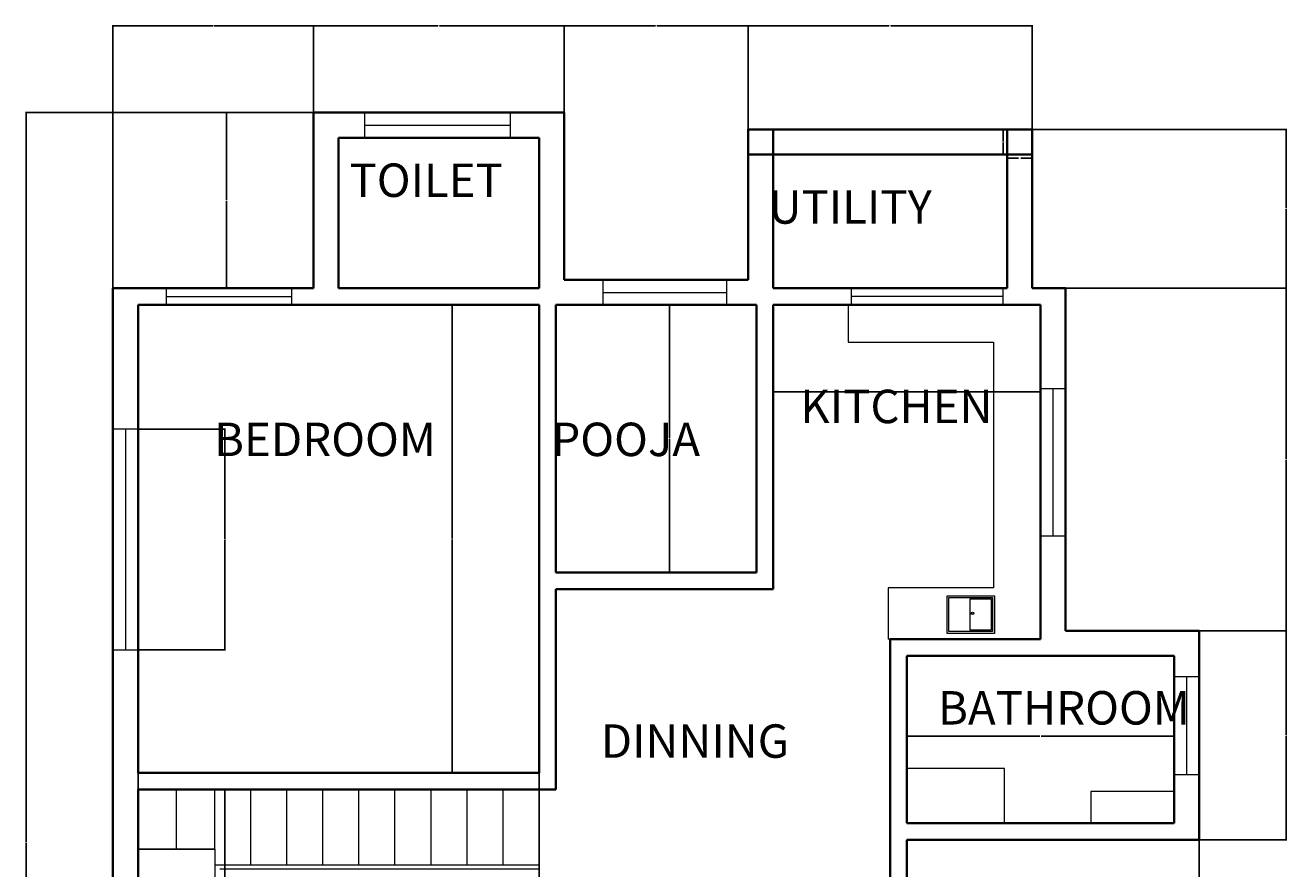
# Model space of a CAD drawing. Units: inches. Extents: x 1741 to 3812, y 9290 to 10023.
# Tile 2 of 5: x 1741 to 2194, y 9630 to 9933. Entities that reach past the tile are written whole.
import ezdxf

# ---------------------------------------------------------------- set-up
doc = ezdxf.new("R2010")
doc.units = ezdxf.units.IN
doc.header["$MEASUREMENT"] = 0
for name, color, linetype, lineweight in [('A-ANNO-DIMS', 2, 'Continuous', 18), ('A-AREA-IDEN', 7, 'Continuous', 18), ('A-COLS', 1, 'Continuous', 35), ('A-FLOR-CASE', 9, 'Continuous', 18), ('A-FLOR-FIXT', 8, 'Continuous', 18), ('A-FLOR-STRS', 3, 'Continuous', 18), ('A-GLAZ', 4, 'Continuous', 18), ('A-WALL', 7, 'Continuous', 35)]:
    doc.layers.add(name, color=color, linetype=linetype, lineweight=lineweight)
doc.styles.get("Standard").update_dxf_attribs({"font": 'arial.ttf'})
doc.dimstyles.get("Standard").update_dxf_attribs({"dimtxt": 0.18, "dimasz": 0.18, "dimexe": 0.18, "dimexo": 0.0625, "dimgap": 0.09, "dimtad": 0, "dimtih": 1, "dimtoh": 1, "dimdec": 4, "dimzin": 0, "dimdsep": 46, "dimtxsty": 'Standard', "dimcen": 0.09, "dimadec": 0, "dimazin": 0, "dimtfac": 1, "dimtdec": 4, "dimtofl": 0, "dimtmove": 0, "dimatfit": 3, "dimfxl": 1, "dimtolj": 1, "dimtzin": 0, "dimarcsym": 0})

# ---------------------------------------------------------------- blocks, each defined once
blk = doc.blocks.new('POST-9X9-PLAN')
blk.add_lwpolyline([(9, 0), (0, 0), (0, 9), (9, 9)], close=True)
blk = doc.blocks.new('*D15')
at = {"layer": 'A-ANNO-DIMS', "color": 0, "lineweight": -2, "transparency": 16777216}
for p, q in [((2093.86, 9895.45), (2092.39, 9895.45)), ((2092.57, 9895.27), (2092.57, 9891.13)), ((2092.57, 9886.63), (2092.57, 9890.77)), ((2093.86, 9886.45), (2092.39, 9886.45))]:
    blk.add_line(p, q, dxfattribs=at)
at = {"layer": 'A-ANNO-DIMS', "color": 0, "transparency": 16777216}
for points in [[(2092.54, 9895.27), (2092.6, 9895.27), (2092.57, 9895.45)], [(2092.54, 9886.63), (2092.6, 9886.63), (2092.57, 9886.45)]]:
    blk.add_solid(points, dxfattribs=at)
at = {"layer": 'Defpoints', "color": 0, "transparency": 16777216}
for p in [(2093.92, 9895.45), (2092.57, 9886.45), (2093.92, 9886.45)]:
    blk.add_point(p, dxfattribs=at)
at = {"layer": 'A-ANNO-DIMS', "color": 0, "transparency": 16777216, "insert": (2092.57, 9890.95), "char_height": 0.18, "attachment_point": 5}
blk.add_mtext('\\A1;POST 9 TYP.', dxfattribs=at)
blk = doc.blocks.new('*D16')
at = {"layer": 'A-ANNO-DIMS', "color": 0, "lineweight": -2, "transparency": 16777216}
for p, q in [((2093.92, 9886.39), (2093.92, 9884.92)), ((2094.1, 9885.1), (2097.97, 9885.1)), ((2102.74, 9885.1), (2098.88, 9885.1)), ((2102.92, 9886.39), (2102.92, 9884.92))]:
    blk.add_line(p, q, dxfattribs=at)
at = {"layer": 'A-ANNO-DIMS', "color": 0, "transparency": 16777216}
for points in [[(2094.1, 9885.13), (2094.1, 9885.07), (2093.92, 9885.1)], [(2102.74, 9885.13), (2102.74, 9885.07), (2102.92, 9885.1)]]:
    blk.add_solid(points, dxfattribs=at)
at = {"layer": 'Defpoints', "color": 0, "transparency": 16777216}
for p in [(2093.92, 9886.45), (2102.92, 9886.45), (2102.92, 9885.1)]:
    blk.add_point(p, dxfattribs=at)
at = {"layer": 'A-ANNO-DIMS', "color": 0, "transparency": 16777216, "insert": (2098.42, 9885.1), "char_height": 0.18, "attachment_point": 5}
blk.add_mtext('\\A1;9 TYP.', dxfattribs=at)
blk = doc.blocks.new('*D31')
at = {"layer": 'A-ANNO-DIMS', "color": 0, "lineweight": -2, "transparency": 16777216}
for p, q in [((2162.92, 9640.39), (2162.92, 9345.97)), ((1772.92, 9391.39), (1772.92, 9345.97)), ((1773.1, 9346.15), (1967.64, 9346.15)), ((2162.74, 9346.15), (1968.21, 9346.15))]:
    blk.add_line(p, q, dxfattribs=at)
at = {"layer": 'A-ANNO-DIMS', "color": 0, "transparency": 16777216}
for points in [[(1773.1, 9346.18), (1773.1, 9346.12), (1772.92, 9346.15)], [(2162.74, 9346.18), (2162.74, 9346.12), (2162.92, 9346.15)]]:
    blk.add_solid(points, dxfattribs=at)
at = {"layer": 'Defpoints', "color": 0, "transparency": 16777216}
for p in [(2162.92, 9640.45), (1772.92, 9391.45), (2162.92, 9346.15)]:
    blk.add_point(p, dxfattribs=at)
at = {"layer": 'A-ANNO-DIMS', "color": 0, "transparency": 16777216, "insert": (1967.92, 9346.15), "char_height": 0.18, "attachment_point": 5}
blk.add_mtext('\\A1;390', dxfattribs=at)
blk = doc.blocks.new('*D32')
at = {"layer": 'A-ANNO-DIMS', "color": 0, "lineweight": -2, "transparency": 16777216}
for p, q in [((1844.86, 9901.45), (1741.54, 9901.45)), ((1741.72, 9901.27), (1741.72, 9639.58)), ((1741.72, 9377.53), (1741.72, 9639.22)), ((1909.43, 9377.35), (1741.54, 9377.35))]:
    blk.add_line(p, q, dxfattribs=at)
at = {"layer": 'A-ANNO-DIMS', "color": 0, "transparency": 16777216}
for points in [[(1741.69, 9901.27), (1741.75, 9901.27), (1741.72, 9901.45)], [(1741.69, 9377.53), (1741.75, 9377.53), (1741.72, 9377.35)]]:
    blk.add_solid(points, dxfattribs=at)
at = {"layer": 'Defpoints', "color": 0, "transparency": 16777216}
for p in [(1741.72, 9901.45), (1844.92, 9901.45), (1909.49, 9377.35)]:
    blk.add_point(p, dxfattribs=at)
at = {"layer": 'A-ANNO-DIMS', "color": 0, "transparency": 16777216, "insert": (1741.72, 9639.4), "char_height": 0.18, "attachment_point": 5}
blk.add_mtext('\\A1;524.1', dxfattribs=at)
blk = doc.blocks.new('*D33')
at = {"layer": 'A-ANNO-DIMS', "color": 0, "lineweight": -2, "transparency": 16777216}
for p, q in [((1772.92, 9838.51), (1772.92, 9932.83)), ((1773.1, 9932.65), (1808.71, 9932.65)), ((1844.74, 9932.65), (1809.14, 9932.65)), ((1844.92, 9838.51), (1844.92, 9932.83))]:
    blk.add_line(p, q, dxfattribs=at)
at = {"layer": 'A-ANNO-DIMS', "color": 0, "transparency": 16777216}
for points in [[(1773.1, 9932.68), (1773.1, 9932.62), (1772.92, 9932.65)], [(1844.74, 9932.68), (1844.74, 9932.62), (1844.92, 9932.65)]]:
    blk.add_solid(points, dxfattribs=at)
at = {"layer": 'Defpoints', "color": 0, "transparency": 16777216}
for p in [(1844.92, 9932.65), (1772.92, 9838.45), (1844.92, 9838.45)]:
    blk.add_point(p, dxfattribs=at)
at = {"layer": 'A-ANNO-DIMS', "color": 0, "transparency": 16777216, "insert": (1808.92, 9932.65), "char_height": 0.18, "attachment_point": 5}
blk.add_mtext('\\A1;72', dxfattribs=at)
blk = doc.blocks.new('*D34')
at = {"layer": 'A-ANNO-DIMS', "color": 0, "lineweight": -2, "transparency": 16777216}
for p, q in [((1844.92, 9901.51), (1844.92, 9932.83)), ((1845.1, 9932.65), (1889.71, 9932.65)), ((1934.74, 9932.65), (1890.14, 9932.65)), ((1934.92, 9901.51), (1934.92, 9932.83))]:
    blk.add_line(p, q, dxfattribs=at)
at = {"layer": 'A-ANNO-DIMS', "color": 0, "transparency": 16777216}
for points in [[(1845.1, 9932.68), (1845.1, 9932.62), (1844.92, 9932.65)], [(1934.74, 9932.68), (1934.74, 9932.62), (1934.92, 9932.65)]]:
    blk.add_solid(points, dxfattribs=at)
at = {"layer": 'Defpoints', "color": 0, "transparency": 16777216}
for p in [(1934.92, 9932.65), (1844.92, 9901.45), (1934.92, 9901.45)]:
    blk.add_point(p, dxfattribs=at)
at = {"layer": 'A-ANNO-DIMS', "color": 0, "transparency": 16777216, "insert": (1889.92, 9932.65), "char_height": 0.18, "attachment_point": 5}
blk.add_mtext('\\A1;90', dxfattribs=at)
blk = doc.blocks.new('*D35')
at = {"layer": 'A-ANNO-DIMS', "color": 0, "lineweight": -2, "transparency": 16777216}
for p, q in [((1934.92, 9841.51), (1934.92, 9932.83)), ((1935.1, 9932.65), (1967.7, 9932.65)), ((2000.74, 9932.65), (1968.14, 9932.65)), ((2000.92, 9841.51), (2000.92, 9932.83))]:
    blk.add_line(p, q, dxfattribs=at)
at = {"layer": 'A-ANNO-DIMS', "color": 0, "transparency": 16777216}
for points in [[(1935.1, 9932.68), (1935.1, 9932.62), (1934.92, 9932.65)], [(2000.74, 9932.68), (2000.74, 9932.62), (2000.92, 9932.65)]]:
    blk.add_solid(points, dxfattribs=at)
at = {"layer": 'Defpoints', "color": 0, "transparency": 16777216}
for p in [(2000.92, 9932.65), (1934.92, 9841.45), (2000.92, 9841.45)]:
    blk.add_point(p, dxfattribs=at)
at = {"layer": 'A-ANNO-DIMS', "color": 0, "transparency": 16777216, "insert": (1967.92, 9932.65), "char_height": 0.18, "attachment_point": 5}
blk.add_mtext('\\A1;66', dxfattribs=at)
blk = doc.blocks.new('*D36')
at = {"layer": 'A-ANNO-DIMS', "color": 0, "lineweight": -2, "transparency": 16777216}
for p, q in [((2000.92, 9895.51), (2000.92, 9932.83)), ((2001.1, 9932.65), (2051.64, 9932.65)), ((2102.74, 9932.65), (2052.2, 9932.65)), ((2102.92, 9895.51), (2102.92, 9932.83))]:
    blk.add_line(p, q, dxfattribs=at)
at = {"layer": 'A-ANNO-DIMS', "color": 0, "transparency": 16777216}
for points in [[(2001.1, 9932.68), (2001.1, 9932.62), (2000.92, 9932.65)], [(2102.74, 9932.68), (2102.74, 9932.62), (2102.92, 9932.65)]]:
    blk.add_solid(points, dxfattribs=at)
at = {"layer": 'Defpoints', "color": 0, "transparency": 16777216}
for p in [(2102.92, 9932.65), (2000.92, 9895.45), (2102.92, 9895.45)]:
    blk.add_point(p, dxfattribs=at)
at = {"layer": 'A-ANNO-DIMS', "color": 0, "transparency": 16777216, "insert": (2051.92, 9932.65), "char_height": 0.18, "attachment_point": 5}
blk.add_mtext('\\A1;102', dxfattribs=at)
blk = doc.blocks.new('*D37')
at = {"layer": 'A-ANNO-DIMS', "color": 0, "lineweight": -2, "transparency": 16777216}
for p, q in [((1844.86, 9901.45), (1813.54, 9901.45)), ((1813.72, 9901.27), (1813.72, 9870.13)), ((1813.72, 9838.63), (1813.72, 9869.77)), ((1844.86, 9838.45), (1813.54, 9838.45))]:
    blk.add_line(p, q, dxfattribs=at)
at = {"layer": 'A-ANNO-DIMS', "color": 0, "transparency": 16777216}
for points in [[(1813.69, 9901.27), (1813.75, 9901.27), (1813.72, 9901.45)], [(1813.69, 9838.63), (1813.75, 9838.63), (1813.72, 9838.45)]]:
    blk.add_solid(points, dxfattribs=at)
at = {"layer": 'Defpoints', "color": 0, "transparency": 16777216}
for p in [(1813.72, 9901.45), (1844.92, 9901.45), (1844.92, 9838.45)]:
    blk.add_point(p, dxfattribs=at)
at = {"layer": 'A-ANNO-DIMS', "color": 0, "transparency": 16777216, "insert": (1813.72, 9869.95), "char_height": 0.18, "attachment_point": 5}
blk.add_mtext('\\A1;63', dxfattribs=at)
blk = doc.blocks.new('*D38')
at = {"layer": 'A-ANNO-DIMS', "color": 0, "lineweight": -2, "transparency": 16777216}
for p, q in [((2102.99, 9895.45), (2194.3, 9895.45)), ((2194.12, 9895.27), (2194.12, 9867.13)), ((2194.12, 9838.63), (2194.12, 9866.77)), ((2102.99, 9838.45), (2194.3, 9838.45))]:
    blk.add_line(p, q, dxfattribs=at)
at = {"layer": 'A-ANNO-DIMS', "color": 0, "transparency": 16777216}
for points in [[(2194.09, 9895.27), (2194.15, 9895.27), (2194.12, 9895.45)], [(2194.09, 9838.63), (2194.15, 9838.63), (2194.12, 9838.45)]]:
    blk.add_solid(points, dxfattribs=at)
at = {"layer": 'Defpoints', "color": 0, "transparency": 16777216}
for p in [(2102.92, 9895.45), (2102.92, 9838.45), (2194.12, 9838.45)]:
    blk.add_point(p, dxfattribs=at)
at = {"layer": 'A-ANNO-DIMS', "color": 0, "transparency": 16777216, "insert": (2194.12, 9866.95), "char_height": 0.18, "attachment_point": 5}
blk.add_mtext('\\A1;57', dxfattribs=at)
blk = doc.blocks.new('*D39')
at = {"layer": 'A-ANNO-DIMS', "color": 0, "lineweight": -2, "transparency": 16777216}
for p, q in [((2114.99, 9838.45), (2194.3, 9838.45)), ((2194.12, 9838.27), (2194.12, 9777.13)), ((2194.12, 9715.63), (2194.12, 9776.77)), ((2114.99, 9715.45), (2194.3, 9715.45))]:
    blk.add_line(p, q, dxfattribs=at)
at = {"layer": 'A-ANNO-DIMS', "color": 0, "transparency": 16777216}
for points in [[(2194.09, 9838.27), (2194.15, 9838.27), (2194.12, 9838.45)], [(2194.09, 9715.63), (2194.15, 9715.63), (2194.12, 9715.45)]]:
    blk.add_solid(points, dxfattribs=at)
at = {"layer": 'Defpoints', "color": 0, "transparency": 16777216}
for p in [(2114.92, 9838.45), (2114.92, 9715.45), (2194.12, 9715.45)]:
    blk.add_point(p, dxfattribs=at)
at = {"layer": 'A-ANNO-DIMS', "color": 0, "transparency": 16777216, "insert": (2194.12, 9776.95), "char_height": 0.18, "attachment_point": 5}
blk.add_mtext('\\A1;123', dxfattribs=at)
blk = doc.blocks.new('*D40')
at = {"layer": 'A-ANNO-DIMS', "color": 0, "lineweight": -2, "transparency": 16777216}
for p, q in [((2162.99, 9715.45), (2194.3, 9715.45)), ((2194.12, 9715.27), (2194.12, 9678.13)), ((2194.12, 9640.63), (2194.12, 9677.77)), ((2162.99, 9640.45), (2194.3, 9640.45))]:
    blk.add_line(p, q, dxfattribs=at)
at = {"layer": 'A-ANNO-DIMS', "color": 0, "transparency": 16777216}
for points in [[(2194.09, 9715.27), (2194.15, 9715.27), (2194.12, 9715.45)], [(2194.09, 9640.63), (2194.15, 9640.63), (2194.12, 9640.45)]]:
    blk.add_solid(points, dxfattribs=at)
at = {"layer": 'Defpoints', "color": 0, "transparency": 16777216}
for p in [(2162.92, 9715.45), (2162.92, 9640.45), (2194.12, 9640.45)]:
    blk.add_point(p, dxfattribs=at)
at = {"layer": 'A-ANNO-DIMS', "color": 0, "transparency": 16777216, "insert": (2194.12, 9677.95), "char_height": 0.18, "attachment_point": 5}
blk.add_mtext('\\A1;75', dxfattribs=at)
blk = doc.blocks.new('*D42')
at = {"layer": 'A-ANNO-DIMS', "color": 0, "lineweight": -2, "transparency": 16777216}
for p, q in [((1781.92, 9832.39), (1781.92, 9345.97)), ((1925.92, 9832.39), (1925.92, 9345.97)), ((1782.1, 9346.15), (1853.64, 9346.15)), ((1925.74, 9346.15), (1854.2, 9346.15))]:
    blk.add_line(p, q, dxfattribs=at)
at = {"layer": 'A-ANNO-DIMS', "color": 0, "transparency": 16777216}
for points in [[(1782.1, 9346.18), (1782.1, 9346.12), (1781.92, 9346.15)], [(1925.74, 9346.18), (1925.74, 9346.12), (1925.92, 9346.15)]]:
    blk.add_solid(points, dxfattribs=at)
at = {"layer": 'Defpoints', "color": 0, "transparency": 16777216}
for p in [(1781.92, 9832.45), (1925.92, 9832.45), (1925.92, 9346.15)]:
    blk.add_point(p, dxfattribs=at)
at = {"layer": 'A-ANNO-DIMS', "color": 0, "transparency": 16777216, "insert": (1853.92, 9346.15), "char_height": 0.18, "attachment_point": 5}
blk.add_mtext('\\A1;144', dxfattribs=at)
blk = doc.blocks.new('*D43')
at = {"layer": 'A-ANNO-DIMS', "color": 0, "lineweight": -2, "transparency": 16777216}
for p, q in [((1925.86, 9832.45), (1894.54, 9832.45)), ((1894.72, 9832.27), (1894.72, 9748.63)), ((1894.72, 9664.63), (1894.72, 9748.27)), ((1925.86, 9664.45), (1894.54, 9664.45))]:
    blk.add_line(p, q, dxfattribs=at)
at = {"layer": 'A-ANNO-DIMS', "color": 0, "transparency": 16777216}
for points in [[(1894.69, 9832.27), (1894.75, 9832.27), (1894.72, 9832.45)], [(1894.69, 9664.63), (1894.75, 9664.63), (1894.72, 9664.45)]]:
    blk.add_solid(points, dxfattribs=at)
at = {"layer": 'Defpoints', "color": 0, "transparency": 16777216}
for p in [(1894.72, 9832.45), (1925.92, 9832.45), (1925.92, 9664.45)]:
    blk.add_point(p, dxfattribs=at)
at = {"layer": 'A-ANNO-DIMS', "color": 0, "transparency": 16777216, "insert": (1894.72, 9748.45), "char_height": 0.18, "attachment_point": 5}
blk.add_mtext('\\A1;168', dxfattribs=at)
blk = doc.blocks.new('*D44')
at = {"layer": 'A-ANNO-DIMS', "color": 0, "lineweight": -2, "transparency": 16777216}
for p, q in [((2003.86, 9832.45), (1972.54, 9832.45)), ((1972.72, 9832.27), (1972.72, 9784.63)), ((1972.72, 9736.63), (1972.72, 9784.27)), ((2003.86, 9736.45), (1972.54, 9736.45))]:
    blk.add_line(p, q, dxfattribs=at)
at = {"layer": 'A-ANNO-DIMS', "color": 0, "transparency": 16777216}
for points in [[(1972.69, 9832.27), (1972.75, 9832.27), (1972.72, 9832.45)], [(1972.69, 9736.63), (1972.75, 9736.63), (1972.72, 9736.45)]]:
    blk.add_solid(points, dxfattribs=at)
at = {"layer": 'Defpoints', "color": 0, "transparency": 16777216}
for p in [(1972.72, 9832.45), (2003.92, 9832.45), (2003.92, 9736.45)]:
    blk.add_point(p, dxfattribs=at)
at = {"layer": 'A-ANNO-DIMS', "color": 0, "transparency": 16777216, "insert": (1972.72, 9784.45), "char_height": 0.18, "attachment_point": 5}
blk.add_mtext('\\A1;96', dxfattribs=at)
blk = doc.blocks.new('*D45')
at = {"layer": 'A-ANNO-DIMS', "color": 0, "lineweight": -2, "transparency": 16777216}
for p, q in [((2009.92, 9832.39), (2009.92, 9801.07)), ((2105.92, 9832.39), (2105.92, 9801.07)), ((2010.1, 9801.25), (2057.71, 9801.25)), ((2105.74, 9801.25), (2058.14, 9801.25))]:
    blk.add_line(p, q, dxfattribs=at)
at = {"layer": 'A-ANNO-DIMS', "color": 0, "transparency": 16777216}
for points in [[(2010.1, 9801.28), (2010.1, 9801.22), (2009.92, 9801.25)], [(2105.74, 9801.28), (2105.74, 9801.22), (2105.92, 9801.25)]]:
    blk.add_solid(points, dxfattribs=at)
at = {"layer": 'Defpoints', "color": 0, "transparency": 16777216}
for p in [(2009.92, 9832.45), (2105.92, 9832.45), (2009.92, 9801.25)]:
    blk.add_point(p, dxfattribs=at)
at = {"layer": 'A-ANNO-DIMS', "color": 0, "transparency": 16777216, "insert": (2057.92, 9801.25), "char_height": 0.18, "attachment_point": 5}
blk.add_mtext('\\A1;96', dxfattribs=at)
blk = doc.blocks.new('*D46')
at = {"layer": 'A-ANNO-DIMS', "color": 0, "lineweight": -2, "transparency": 16777216}
for p, q in [((2057.92, 9646.51), (2057.92, 9677.83)), ((2058.1, 9677.65), (2105.71, 9677.65)), ((2153.74, 9677.65), (2106.14, 9677.65)), ((2153.92, 9646.51), (2153.92, 9677.83))]:
    blk.add_line(p, q, dxfattribs=at)
at = {"layer": 'A-ANNO-DIMS', "color": 0, "transparency": 16777216}
for points in [[(2058.1, 9677.68), (2058.1, 9677.62), (2057.92, 9677.65)], [(2153.74, 9677.68), (2153.74, 9677.62), (2153.92, 9677.65)]]:
    blk.add_solid(points, dxfattribs=at)
at = {"layer": 'Defpoints', "color": 0, "transparency": 16777216}
for p in [(2153.92, 9677.65), (2057.92, 9646.45), (2153.92, 9646.45)]:
    blk.add_point(p, dxfattribs=at)
at = {"layer": 'A-ANNO-DIMS', "color": 0, "transparency": 16777216, "insert": (2105.92, 9677.65), "char_height": 0.18, "attachment_point": 5}
blk.add_mtext('\\A1;96', dxfattribs=at)
blk = doc.blocks.new('*D48')
at = {"layer": 'A-ANNO-DIMS', "color": 0, "lineweight": -2, "transparency": 16777216}
for p, q in [((1781.99, 9658.45), (1813.3, 9658.45)), ((1813.12, 9658.27), (1813.12, 9574.63)), ((1813.12, 9490.63), (1813.12, 9574.27)), ((1781.99, 9490.45), (1813.3, 9490.45))]:
    blk.add_line(p, q, dxfattribs=at)
at = {"layer": 'A-ANNO-DIMS', "color": 0, "transparency": 16777216}
for points in [[(1813.09, 9658.27), (1813.15, 9658.27), (1813.12, 9658.45)], [(1813.09, 9490.63), (1813.15, 9490.63), (1813.12, 9490.45)]]:
    blk.add_solid(points, dxfattribs=at)
at = {"layer": 'Defpoints', "color": 0, "transparency": 16777216}
for p in [(1781.92, 9658.45), (1781.92, 9490.45), (1813.12, 9490.45)]:
    blk.add_point(p, dxfattribs=at)
at = {"layer": 'A-ANNO-DIMS', "color": 0, "transparency": 16777216, "insert": (1813.12, 9574.45), "char_height": 0.18, "attachment_point": 5}
blk.add_mtext('\\A1;168', dxfattribs=at)
blk = doc.blocks.new('*D52')
at = {"layer": 'A-ANNO-DIMS', "color": 0, "lineweight": -2, "transparency": 16777216}
for p, q in [((1781.99, 9787.82), (1813.3, 9787.82)), ((1813.12, 9787.64), (1813.12, 9748.39)), ((1813.12, 9708.79), (1813.12, 9748.03)), ((1781.99, 9708.61), (1813.3, 9708.61))]:
    blk.add_line(p, q, dxfattribs=at)
at = {"layer": 'A-ANNO-DIMS', "color": 0, "transparency": 16777216}
for points in [[(1813.09, 9787.64), (1813.15, 9787.64), (1813.12, 9787.82)], [(1813.09, 9708.79), (1813.15, 9708.79), (1813.12, 9708.61)]]:
    blk.add_solid(points, dxfattribs=at)
at = {"layer": 'Defpoints', "color": 0, "transparency": 16777216}
for p in [(1781.92, 9787.82), (1781.92, 9708.61), (1813.12, 9708.61)]:
    blk.add_point(p, dxfattribs=at)
at = {"layer": 'A-ANNO-DIMS', "color": 0, "transparency": 16777216, "insert": (1813.12, 9748.21), "char_height": 0.18, "attachment_point": 5}
blk.add_mtext('\\A1;79.2', dxfattribs=at)

msp = doc.modelspace()

# ---------------------------------------------------------------- linework, layer by layer
at = {"layer": 'A-FLOR-CASE'}
for p, q in [((2036.8766, 9832.4507), (2036.8766, 9819.0994)), ((2036.8766, 9819.0994), (2089.0781, 9819.0994)), ((2089.0781, 9819.0994), (2089.0781, 9730.9078)), ((2089.0781, 9730.9078), (2051.2639, 9730.9078)), ((2051.2639, 9730.9078), (2051.2639, 9712.4507)), ((2051.9242, 9712.4507), (2051.2639, 9712.4507))]:
    msp.add_line(p, q, dxfattribs=at)
at = {"layer": 'A-FLOR-FIXT'}
for points in [[(2072.355, 9728.0439), (2089.4179, 9728.0439), (2089.4179, 9714.5101), (2072.355, 9714.5101)], [(2073.032, 9727.367), (2088.741, 9727.367), (2088.741, 9715.187), (2073.032, 9715.187)], [(2080.6059, 9726.9568), (2088.2516, 9726.9568), (2088.2516, 9715.6459), (2080.6059, 9715.6459)], [(2057.9242, 9646.4507), (2092.9706, 9646.4507), (2092.9706, 9666.0969), (2057.9242, 9666.0969)], [(2153.9242, 9657.8019), (2124.0009, 9657.8019), (2124.0009, 9646.4507), (2153.9242, 9646.4507)]]:
    msp.add_lwpolyline(points, close=True, dxfattribs=at)
for radius in [0.4264, 0.388]:
    msp.add_circle((2081.5019, 9721.7043), radius, dxfattribs=at)
at = {"layer": 'A-FLOR-STRS'}
for p, q in [((1795.6863, 9637.0717), (1795.6863, 9658.4507)), ((1809.4485, 9637.0717), (1809.4485, 9658.4507)), ((1822.3902, 9631.5196), (1822.3902, 9658.4507)), ((1835.332, 9631.5196), (1835.332, 9658.4507)), ((1848.2737, 9631.5196), (1848.2737, 9658.4507)), ((1861.2155, 9631.5196), (1861.2155, 9658.4507)), ((1874.1572, 9631.5196), (1874.1572, 9658.4507)), ((1887.0989, 9631.5196), (1887.0989, 9658.4507)), ((1900.0407, 9631.5196), (1900.0407, 9658.4507)), ((1912.9824, 9631.5196), (1912.9824, 9658.4507)), ((1925.9242, 9658.4507), (1925.9242, 9630.0587)), ((1925.9242, 9635.2749), (1925.9242, 9658.4507)), ((1809.4485, 9637.0717), (1781.9242, 9637.0717)), ((1781.9242, 9637.0717), (1809.4485, 9637.0717)), ((1809.4485, 9637.0717), (1809.4485, 9561.6958)), ((1809.4485, 9631.5196), (1925.9242, 9631.5196)), ((1811.2454, 9630.0587), (1925.9242, 9630.0587))]:
    msp.add_line(p, q, dxfattribs=at)
at = {"layer": 'A-GLAZ'}
for p, q in [((1863.3847, 9896.9507), (1915.4639, 9896.9507)), ((1792.1334, 9835.4507), (1837.0589, 9835.4507)), ((1948.8543, 9836.9507), (1993.1419, 9836.9507)), ((2092.4003, 9835.4507), (2038.0681, 9835.4507)), ((2110.4242, 9749.5281), (2110.4242, 9802.3044)), ((1777.4242, 9787.815), (1777.4242, 9708.6102)), ((2158.4242, 9663.8403), (2158.4242, 9698.9294))]:
    msp.add_line(p, q, dxfattribs=at)
for points in [[(1863.3847, 9901.4507), (1915.4639, 9901.4507), (1915.4639, 9892.4507), (1863.3847, 9892.4507)], [(1792.1334, 9838.4507), (1837.0589, 9838.4507), (1837.0589, 9832.4507), (1792.1334, 9832.4507)], [(1948.8543, 9841.4507), (1993.1419, 9841.4507), (1993.1419, 9832.4507), (1948.8543, 9832.4507)], [(2038.0681, 9838.4507), (2092.4003, 9838.4507), (2092.4003, 9832.4507), (2038.0681, 9832.4507)], [(2114.9242, 9802.3044), (2105.9242, 9802.3044), (2105.9242, 9749.5281), (2114.9242, 9749.5281)], [(1781.9242, 9787.815), (1772.9242, 9787.815), (1772.9242, 9708.6102), (1781.9242, 9708.6102)], [(2162.9242, 9698.9294), (2153.9242, 9698.9294), (2153.9242, 9663.8403), (2162.9242, 9663.8403)]]:
    msp.add_lwpolyline(points, close=True, dxfattribs=at)
at = {"layer": 'A-WALL'}
for p, q in [((1934.9242, 9901.4507), (1844.9242, 9901.4507)), ((1844.9242, 9901.4507), (1844.9242, 9838.4507)), ((1934.9242, 9841.4507), (1934.9242, 9901.4507)), ((1925.9242, 9892.4507), (1853.9242, 9892.4507)), ((1853.9242, 9892.4507), (1853.9242, 9838.4507)), ((1925.9242, 9838.4507), (1925.9242, 9892.4507)), ((2000.9242, 9895.4507), (2102.9242, 9895.4507)), ((2000.9242, 9841.4507), (2000.9242, 9895.4507)), ((2102.9242, 9895.4507), (2102.9242, 9838.4507)), ((2009.9242, 9838.4507), (2009.9242, 9886.4507)), ((2009.9242, 9886.4507), (2093.9242, 9886.4507)), ((2093.9242, 9886.4507), (2093.9242, 9838.4507)), ((1781.9242, 9838.4507), (1772.9242, 9838.4507)), ((1772.9242, 9832.4507), (1772.9242, 9838.4507)), ((1781.9242, 9838.4507), (1844.9242, 9838.4507)), ((1853.9242, 9838.4507), (1925.9242, 9838.4507)), ((1934.9242, 9841.4507), (2000.9242, 9841.4507)), ((2009.9242, 9838.4507), (2093.9242, 9838.4507)), ((2102.9242, 9838.4507), (2105.9242, 9838.4507)), ((2105.9242, 9838.4507), (2114.9242, 9838.4507)), ((2114.9242, 9832.4507), (2114.9242, 9838.4507)), ((1772.9242, 9664.4507), (1772.9242, 9832.4507)), ((1781.9242, 9832.4507), (1925.9242, 9832.4507)), ((1781.9242, 9664.4507), (1781.9242, 9832.4507)), ((1925.9242, 9832.4507), (1925.9242, 9664.4507)), ((1931.9242, 9832.4507), (1931.9242, 9736.4507)), ((1931.9242, 9832.4507), (2003.9242, 9832.4507)), ((2003.9242, 9832.4507), (2003.9242, 9736.4507)), ((2009.9242, 9832.4507), (2009.9242, 9730.4507)), ((2009.9242, 9832.4507), (2105.9242, 9832.4507)), ((2105.9242, 9832.4507), (2105.9242, 9712.4507)), ((2114.9242, 9832.4507), (2114.9242, 9715.4507)), ((2003.9242, 9736.4507), (1931.9242, 9736.4507)), ((1925.9242, 9730.4507), (1925.9242, 9664.4507)), ((2009.9242, 9730.4507), (1931.9242, 9730.4507)), ((1931.9242, 9730.4507), (1931.9242, 9658.4507)), ((1931.9242, 9730.4507), (1931.9242, 9664.4507)), ((2162.9242, 9715.4507), (2114.9242, 9715.4507)), ((2162.9242, 9640.4507), (2162.9242, 9715.4507)), ((2051.9242, 9610.4507), (2051.9242, 9712.4507)), ((2105.9242, 9712.4507), (2051.9242, 9712.4507)), ((2153.9242, 9706.4507), (2057.9242, 9706.4507)), ((2057.9242, 9646.4507), (2057.9242, 9706.4507)), ((2153.9242, 9646.4507), (2153.9242, 9706.4507)), ((1772.9242, 9664.4507), (1772.9242, 9658.4507)), ((1925.9242, 9664.4507), (1781.9242, 9664.4507)), ((1772.9242, 9658.4507), (1772.9242, 9490.4507)), ((1931.9242, 9658.4507), (1781.9242, 9658.4507)), ((1781.9242, 9658.4507), (1781.9242, 9490.4507)), ((2153.9242, 9646.4507), (2057.9242, 9646.4507)), ((2057.9242, 9613.4507), (2057.9242, 9640.4507)), ((2162.9242, 9640.4507), (2057.9242, 9640.4507))]:
    msp.add_line(p, q, dxfattribs=at)

# ---------------------------------------------------------------- block references
at = {"layer": 'A-COLS'}
msp.add_blockref('POST-9X9-PLAN', (2000.924, 9886.451), dxfattribs=at)
at = {"layer": 'A-COLS', "rotation": 269.9999999999952}
msp.add_blockref('POST-9X9-PLAN', (2093.9245, 9895.4509), dxfattribs=at)

# ---------------------------------------------------------------- texts
at = {"layer": 'A-AREA-IDEN'}
for s, p in [('TOILET', (1857.8217, 9871.2015)), ('UTILITY', (2008.3136, 9861.6028)), ('KITCHEN', (2019.6689, 9790.005)), ('BEDROOM', (1809.2067, 9778.1769)), ('POOJA  ', (1930.3191, 9778.1769)), ('BATHROOM ', (2069.1196, 9681.8229)), ('DINNING', (1948.0256, 9669.8934))]:
    msp.add_text(s, height=12, dxfattribs=at).set_placement(p)

# ---------------------------------------------------------------- dimensions: what is measured, and where the dimension line sits
at = {"layer": 'A-ANNO-DIMS'}
for base, p1, p2, picture, middle in [((1844.9242, 9932.6507), (1772.9242, 9838.4507), (1844.9242, 9838.4507), '*D33', (1808.9242, 9932.6507)), ((1934.9242, 9932.6507), (1844.9242, 9901.4507), (1934.9242, 9901.4507), '*D34', (1889.9242, 9932.6507)), ((2000.9242, 9932.6507), (1934.9242, 9841.4507), (2000.9242, 9841.4507), '*D35', (1967.9242, 9932.6507)), ((2102.9242, 9932.6507), (2000.9242, 9895.4507), (2102.9242, 9895.4507), '*D36', (2051.9242, 9932.6507)), ((1925.9242, 9346.1522), (1781.9242, 9832.4507), (1925.9242, 9832.4507), '*D42', (1853.9242, 9346.1522)), ((2153.9242, 9677.6507), (2057.9242, 9646.4507), (2153.9242, 9646.4507), '*D46', (2105.9242, 9677.6507)), ((2162.9242, 9346.1522), (1772.9242, 9391.4507), (2162.9242, 9640.4507), '*D31', (1967.9242, 9346.1522))]:
    dim = msp.add_linear_dim(base=base, p1=p1, p2=p2, dimstyle='Standard', override={"dimdec": 0, "dimlfac": 1, "dimrnd": 0, "dimzin": 0, "dimdsep": 46, "dimlunit": 2}, dxfattribs=at)
    dim.commit()
    dim.dimension.update_dxf_attribs({"geometry": picture, "text_midpoint": middle})
for base, p1, p2, angle, override, picture, middle in [((1741.7242, 9901.4507), (1909.4893, 9377.3522), (1844.9242, 9901.4507), 90, {"dimdec": 1, "dimlfac": 1, "dimrnd": 0, "dimzin": 0, "dimdsep": 46, "dimlunit": 2}, '*D32', (1741.7242, 9639.4015)), ((1813.7242, 9901.4507), (1844.9242, 9838.4507), (1844.9242, 9901.4507), 90, {"dimdec": 0, "dimlfac": 1, "dimrnd": 0, "dimzin": 0, "dimdsep": 46, "dimlunit": 2}, '*D37', (1813.7242, 9869.9507)), ((2194.1242, 9838.4507), (2102.9242, 9895.4507), (2102.9242, 9838.4507), 90, {"dimdec": 0, "dimlfac": 1, "dimrnd": 0, "dimzin": 0, "dimdsep": 46, "dimlunit": 2}, '*D38', (2194.1242, 9866.9507)), ((2194.1242, 9715.4507), (2114.9242, 9838.4507), (2114.9242, 9715.4507), 90, {"dimdec": 0, "dimlfac": 1, "dimrnd": 0, "dimzin": 0, "dimdsep": 46, "dimlunit": 2}, '*D39', (2194.1242, 9776.9507)), ((1894.7242, 9832.4507), (1925.9242, 9664.4507), (1925.9242, 9832.4507), 90, {"dimdec": 0, "dimlfac": 1, "dimrnd": 0, "dimzin": 0, "dimdsep": 46, "dimlunit": 2}, '*D43', (1894.7242, 9748.4507)), ((1972.7242, 9832.4507), (2003.9242, 9736.4507), (2003.9242, 9832.4507), 90, {"dimdec": 0, "dimlfac": 1, "dimrnd": 0, "dimzin": 0, "dimdsep": 46, "dimlunit": 2}, '*D44', (1972.7242, 9784.4507)), ((2009.9242, 9801.2507), (2105.9242, 9832.4507), (2009.9242, 9832.4507), 180, {"dimdec": 0, "dimlfac": 1, "dimrnd": 0, "dimzin": 0, "dimdsep": 46, "dimlunit": 2}, '*D45', (2057.9242, 9801.2507)), ((1813.1242, 9708.6102), (1781.9242, 9787.815), (1781.9242, 9708.6102), 270, {"dimdec": 1, "dimlfac": 1, "dimrnd": 0, "dimzin": 0, "dimdsep": 46, "dimlunit": 2}, '*D52', (1813.1242, 9748.2126)), ((2194.1242, 9640.4507), (2162.9242, 9715.4507), (2162.9242, 9640.4507), 90, {"dimdec": 0, "dimlfac": 1, "dimrnd": 0, "dimzin": 0, "dimdsep": 46, "dimlunit": 2}, '*D40', (2194.1242, 9677.9507)), ((1813.1242, 9490.4507), (1781.9242, 9658.4507), (1781.9242, 9490.4507), 270, {"dimdec": 0, "dimlfac": 1, "dimrnd": 0, "dimzin": 0, "dimdsep": 46, "dimlunit": 2}, '*D48', (1813.1242, 9574.4507))]:
    dim = msp.add_linear_dim(base=base, p1=p1, p2=p2, angle=angle, dimstyle='Standard', override=override, dxfattribs=at)
    dim.commit()
    dim.dimension.update_dxf_attribs({"geometry": picture, "text_midpoint": middle})
dim = msp.add_linear_dim(base=(2092.5742, 9886.4507), p1=(2093.9242, 9895.4507), p2=(2093.9242, 9886.4507), angle=270, text='POST <> TYP.', dimstyle='Standard', override={"dimdec": 0, "dimlfac": 1, "dimrnd": 0, "dimzin": 0, "dimdsep": 46, "dimlunit": 2}, dxfattribs=at)
dim.commit()
dim.dimension.update_dxf_attribs({"geometry": '*D15', "text_midpoint": (2092.5742, 9890.9507)})
dim = msp.add_linear_dim(base=(2102.9242, 9885.1007), p1=(2093.9242, 9886.4507), p2=(2102.9242, 9886.4507), text='<> TYP.', dimstyle='Standard', override={"dimdec": 0, "dimlfac": 1, "dimrnd": 0, "dimzin": 0, "dimdsep": 46, "dimlunit": 2}, dxfattribs=at)
dim.commit()
dim.dimension.update_dxf_attribs({"geometry": '*D16', "text_midpoint": (2098.4242, 9885.1007)})

doc.saveas('drawing.dxf')
